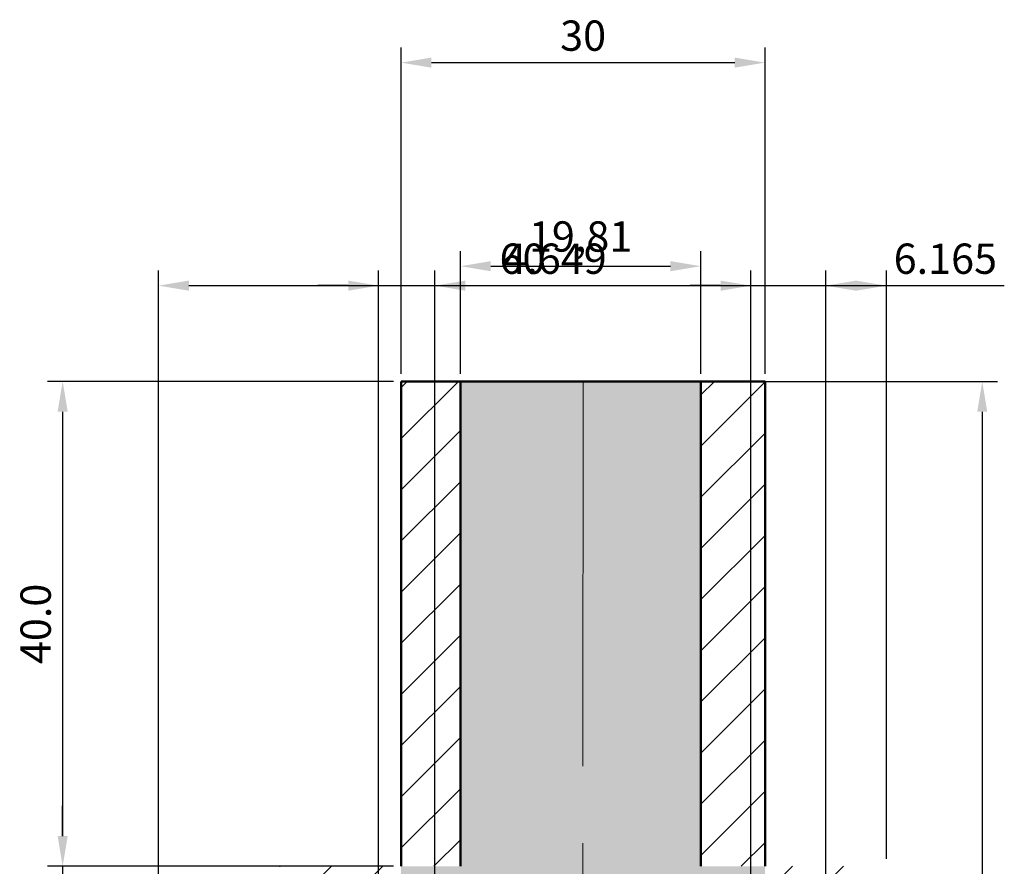
# Model space of a CAD drawing. Units: millimetres. Extents: x 1159 to 1466, y 1237 to 1440.
# Tile 6 of 6: x 1378 to 1459, y 1336 to 1405. Entities that reach past the tile are written whole.
import ezdxf

# ---------------------------------------------------------------- set-up
doc = ezdxf.new("R2010")
doc.units = ezdxf.units.MM
doc.linetypes.add('CENTER', pattern=[50.8, 31.75, -6.35, 6.35, -6.35])
for name, color, linetype, lineweight in [('M-CNTR', 1, 'CENTER', 18), ('M-DIMS', 2, 'Continuous', 25), ('M-HATC', 8, 'Continuous', 18), ('M-OUTL', 7, 'Continuous', 50)]:
    doc.layers.add(name, color=color, linetype=linetype, lineweight=lineweight)
doc.styles.get("Standard").update_dxf_attribs({"font": 'arial.ttf'})
doc.dimstyles.new('ISO-25', dxfattribs={"dimtxt": 2.5, "dimasz": 2.5, "dimexe": 1.25, "dimexo": 0.625, "dimtad": 1, "dimtxsty": 'Standard', "dimcen": 2.5, "dimadec": 0, "dimazin": 0, "dimtfac": 1, "dimtmove": 0, "dimatfit": 3, "dimfxl": 1, "dimarcsym": 0})

# ---------------------------------------------------------------- blocks, each defined once
blk = doc.blocks.new('*D20')
at = {"layer": 'Defpoints', "color": 0, "transparency": 16777216}
for p in [(1439.751, 1401.86), (1409.751, 1375.561), (1439.751, 1375.561)]:
    blk.add_point(p, dxfattribs=at)
at = {"layer": 'M-DIMS', "color": 0, "lineweight": -2, "transparency": 16777216}
for p, q in [((1409.751, 1376.186), (1409.751, 1403.11)), ((1439.751, 1376.186), (1439.751, 1403.11)), ((1412.251, 1401.86), (1437.251, 1401.86))]:
    blk.add_line(p, q, dxfattribs=at)
at = {"layer": 'M-DIMS', "color": 0, "transparency": 16777216}
for points in [[(1412.251, 1402.277), (1412.251, 1401.443), (1409.751, 1401.86)], [(1437.251, 1402.277), (1437.251, 1401.443), (1439.751, 1401.86)]]:
    blk.add_solid(points, dxfattribs=at)
at = {"layer": 'M-DIMS', "color": 0, "transparency": 16777216, "insert": (1424.751, 1403.762), "char_height": 2.5, "attachment_point": 5}
blk.add_mtext('30', dxfattribs=at)
blk = doc.blocks.new('*D21')
at = {"layer": 'Defpoints', "color": 0, "transparency": 16777216}
for p in [(1434.452, 1385.066), (1414.637, 1375.561), (1434.452, 1375.561)]:
    blk.add_point(p, dxfattribs=at)
at = {"layer": 'M-DIMS', "color": 0, "lineweight": -2, "transparency": 16777216}
for p, q in [((1414.637, 1376.186), (1414.637, 1386.316)), ((1434.452, 1376.186), (1434.452, 1386.316)), ((1417.137, 1385.066), (1431.952, 1385.066))]:
    blk.add_line(p, q, dxfattribs=at)
at = {"layer": 'M-DIMS', "color": 0, "transparency": 16777216}
for points in [[(1417.137, 1385.483), (1417.137, 1384.649), (1414.637, 1385.066)], [(1431.952, 1385.483), (1431.952, 1384.649), (1434.452, 1385.066)]]:
    blk.add_solid(points, dxfattribs=at)
at = {"layer": 'M-DIMS', "color": 0, "transparency": 16777216, "insert": (1424.544, 1387.193), "char_height": 2.5, "attachment_point": 5}
blk.add_mtext('19,81', dxfattribs=at)
blk = doc.blocks.new('*D42')
at = {"layer": 'Defpoints', "color": 0, "transparency": 16777216}
for p in [(1409.751, 1375.561), (1424.964, 1255.799), (1457.651, 1255.799)]:
    blk.add_point(p, dxfattribs=at)
at = {"layer": 'M-DIMS', "color": 0, "lineweight": -2, "transparency": 16777216}
for p, q in [((1410.376, 1375.561), (1458.901, 1375.561)), ((1457.651, 1373.061), (1457.651, 1258.299)), ((1425.589, 1255.799), (1458.901, 1255.799))]:
    blk.add_line(p, q, dxfattribs=at)
at = {"layer": 'M-DIMS', "color": 0, "transparency": 16777216}
for points in [[(1457.234, 1373.061), (1458.067, 1373.061), (1457.651, 1375.561)], [(1457.234, 1258.299), (1458.067, 1258.299), (1457.651, 1255.799)]]:
    blk.add_solid(points, dxfattribs=at)
at = {"layer": 'M-DIMS', "color": 0, "transparency": 16777216, "insert": (1455.749, 1315.68), "char_height": 2.5, "attachment_point": 5, "rotation": 90}
blk.add_mtext('119.76', dxfattribs=at)
blk = doc.blocks.new('*D43')
at = {"layer": 'Defpoints', "color": 0, "transparency": 16777216}
for p in [(1449.751, 1383.461), (1449.751, 1335.561), (1389.751, 1330.561)]:
    blk.add_point(p, dxfattribs=at)
at = {"layer": 'M-DIMS', "color": 0, "lineweight": -2, "transparency": 16777216}
for p, q in [((1389.751, 1331.186), (1389.751, 1384.711)), ((1449.751, 1336.186), (1449.751, 1384.711)), ((1392.251, 1383.461), (1447.251, 1383.461))]:
    blk.add_line(p, q, dxfattribs=at)
at = {"layer": 'M-DIMS', "color": 0, "transparency": 16777216}
for points in [[(1392.251, 1383.878), (1392.251, 1383.044), (1389.751, 1383.461)], [(1447.251, 1383.878), (1447.251, 1383.044), (1449.751, 1383.461)]]:
    blk.add_solid(points, dxfattribs=at)
at = {"layer": 'M-DIMS', "color": 0, "transparency": 16777216, "insert": (1419.751, 1385.362), "char_height": 2.5, "attachment_point": 5}
blk.add_mtext('60', dxfattribs=at)
blk = doc.blocks.new('*D57')
at = {"layer": 'Defpoints', "color": 0, "transparency": 16777216}
for p in [(1409.751, 1375.561), (1381.851, 1335.561), (1409.751, 1335.561)]:
    blk.add_point(p, dxfattribs=at)
at = {"layer": 'M-DIMS', "color": 0, "lineweight": -2, "transparency": 16777216}
for p, q in [((1409.126, 1375.561), (1380.601, 1375.561)), ((1381.851, 1373.061), (1381.851, 1338.061)), ((1409.126, 1335.561), (1380.601, 1335.561))]:
    blk.add_line(p, q, dxfattribs=at)
at = {"layer": 'M-DIMS', "color": 0, "transparency": 16777216}
for points in [[(1381.434, 1373.061), (1382.267, 1373.061), (1381.851, 1375.561)], [(1381.434, 1338.061), (1382.267, 1338.061), (1381.851, 1335.561)]]:
    blk.add_solid(points, dxfattribs=at)
at = {"layer": 'M-DIMS', "color": 0, "transparency": 16777216, "insert": (1379.949, 1355.561), "char_height": 2.5, "attachment_point": 5, "rotation": 90}
blk.add_mtext('40.0', dxfattribs=at)
blk = doc.blocks.new('*D58')
at = {"layer": 'Defpoints', "color": 0, "transparency": 16777216}
for p in [(1399.751, 1335.561), (1381.851, 1330.561), (1389.751, 1330.561)]:
    blk.add_point(p, dxfattribs=at)
at = {"layer": 'M-DIMS', "color": 0, "lineweight": -2, "transparency": 16777216}
for p, q in [((1381.851, 1338.061), (1381.851, 1340.561)), ((1399.126, 1335.561), (1380.601, 1335.561)), ((1381.851, 1335.561), (1381.851, 1330.561)), ((1389.126, 1330.561), (1380.601, 1330.561)), ((1381.851, 1328.061), (1381.851, 1319.768))]:
    blk.add_line(p, q, dxfattribs=at)
at = {"layer": 'M-DIMS', "color": 0, "transparency": 16777216}
for points in [[(1381.434, 1338.061), (1382.267, 1338.061), (1381.851, 1335.561)], [(1381.434, 1328.061), (1382.267, 1328.061), (1381.851, 1330.561)]]:
    blk.add_solid(points, dxfattribs=at)
at = {"layer": 'M-DIMS', "color": 0, "transparency": 16777216, "insert": (1379.949, 1322.665), "char_height": 2.5, "attachment_point": 5, "rotation": 90}
blk.add_mtext('5.0', dxfattribs=at)
blk = doc.blocks.new('*D74')
at = {"layer": 'Defpoints', "color": 0, "transparency": 16777216}
for p in [(1412.534, 1383.461), (1407.885, 1271.665), (1412.534, 1264.983)]:
    blk.add_point(p, dxfattribs=at)
at = {"layer": 'M-DIMS', "color": 0, "lineweight": -2, "transparency": 16777216}
for p, q in [((1407.885, 1272.29), (1407.885, 1384.711)), ((1412.534, 1265.608), (1412.534, 1384.711)), ((1405.385, 1383.461), (1402.885, 1383.461)), ((1407.885, 1383.461), (1412.534, 1383.461)), ((1415.034, 1383.461), (1427.326, 1383.461))]:
    blk.add_line(p, q, dxfattribs=at)
at = {"layer": 'M-DIMS', "color": 0, "transparency": 16777216}
for points in [[(1405.385, 1383.878), (1405.385, 1383.044), (1407.885, 1383.461)], [(1415.034, 1383.878), (1415.034, 1383.044), (1412.534, 1383.461)]]:
    blk.add_solid(points, dxfattribs=at)
at = {"layer": 'M-DIMS', "color": 0, "transparency": 16777216, "insert": (1422.43, 1385.362), "char_height": 2.5, "attachment_point": 5}
blk.add_mtext('4.649', dxfattribs=at)
blk = doc.blocks.new('*D75')
at = {"layer": 'Defpoints', "color": 0, "transparency": 16777216}
for p in [(1444.751, 1383.461), (1444.751, 1270.561), (1438.586, 1264.983)]:
    blk.add_point(p, dxfattribs=at)
at = {"layer": 'M-DIMS', "color": 0, "lineweight": -2, "transparency": 16777216}
for p, q in [((1438.586, 1265.608), (1438.586, 1384.711)), ((1444.751, 1271.186), (1444.751, 1384.711)), ((1436.086, 1383.461), (1433.586, 1383.461)), ((1438.586, 1383.461), (1444.751, 1383.461)), ((1447.251, 1383.461), (1459.469, 1383.461))]:
    blk.add_line(p, q, dxfattribs=at)
at = {"layer": 'M-DIMS', "color": 0, "transparency": 16777216}
for points in [[(1436.086, 1383.878), (1436.086, 1383.044), (1438.586, 1383.461)], [(1447.251, 1383.878), (1447.251, 1383.044), (1444.751, 1383.461)]]:
    blk.add_solid(points, dxfattribs=at)
at = {"layer": 'M-DIMS', "color": 0, "transparency": 16777216, "insert": (1454.61, 1385.362), "char_height": 2.5, "attachment_point": 5}
blk.add_mtext('6.165', dxfattribs=at)

msp = doc.modelspace()

# ---------------------------------------------------------------- hatches: boundary and pattern name
at = {"layer": 'M-HATC'}
h = msp.add_hatch(dxfattribs=at)
h.set_pattern_fill('ANSI31', color=256, scale=0.94)
h.set_pattern_definition([(45, (0, -76.8912), (-2.11036, 2.11036), [])])
h.paths.add_polyline_path([(1414.6374, 1375.561), (1409.7508, 1375.561), (1409.7508, 1335.561), (1414.6374, 1335.561)])
h.paths.add_polyline_path([(1439.7508, 1375.561), (1434.4515, 1375.561), (1434.4515, 1335.561), (1439.7508, 1335.561)])
h.paths.add_polyline_path([(1449.7508, 1315.561), (1444.7508, 1315.561), (1444.7508, 1320.561), (1449.7508, 1320.561), (1449.7508, 1335.561), (1439.7508, 1335.561), (1439.7508, 1320.561), (1429.7508, 1320.561), (1429.7508, 1317.561), (1434.7508, 1317.561), (1434.7508, 1282.561), (1429.7508, 1282.561), (1429.7508, 1267.561, -0.1562704), (1427.7989, 1264.9827), (1438.5857, 1264.9827), (1444.7508, 1270.561), (1444.7508, 1275.561), (1444.7508, 1295.561), (1449.7508, 1295.561)])
h.paths.add_polyline_path([(1414.7508, 1317.561), (1419.7508, 1317.561), (1419.7508, 1320.561), (1409.7508, 1320.561), (1409.7508, 1335.561), (1399.7508, 1335.561), (1399.7508, 1330.561), (1389.7508, 1330.561), (1389.7508, 1320.561), (1399.7508, 1320.561), (1399.7508, 1315.561), (1404.7508, 1315.561), (1407.8849, 1311.6652), (1407.8849, 1301.6652), (1402.8849, 1301.6652), (1402.8849, 1281.6652), (1407.8849, 1281.6652), (1407.8849, 1271.6652), (1412.5343, 1264.9827), (1421.7027, 1264.9827, -0.1562704), (1419.7508, 1267.561), (1419.7508, 1282.561), (1414.7508, 1282.561)])
h.paths.add_polyline_path([(1424.6651, 1264.0191, -0.1502665), (1421.7027, 1264.9827), (1412.5343, 1264.9827), (1415.9205, 1260.1158, 0.2337513), (1424.6588, 1255.7945)])
h.paths.add_polyline_path([(1433.7538, 1260.6108), (1438.5857, 1264.9827), (1427.7989, 1264.9827, -0.1585441), (1424.6651, 1264.0191), (1424.6588, 1255.7945, 0.248431)])
h = msp.add_hatch(color=256, dxfattribs=at)
h.set_gradient(color1=(34, 52, 110), color2=(0, 0, 0))
h.paths.add_polyline_path([(1424.7508, 1375.561), (1414.6374, 1375.561), (1414.6374, 1335.561), (1424.7201, 1335.561)])
h.paths.add_polyline_path([(1434.4515, 1375.561), (1424.7508, 1375.561), (1424.7201, 1335.561), (1434.4515, 1335.561)])
h.paths.add_polyline_path([(1424.7201, 1335.561), (1414.6374, 1335.561), (1409.7508, 1335.561), (1409.7508, 1320.561), (1424.7085, 1320.561)])
h.paths.add_polyline_path([(1439.7508, 1335.561), (1424.7201, 1335.561), (1424.7085, 1320.561), (1424.7508, 1320.561), (1439.7508, 1320.561)])
h.paths.add_polyline_path([(1434.7508, 1317.561), (1429.7508, 1317.561), (1424.7062, 1317.561), (1424.6793, 1282.561), (1424.7508, 1282.561), (1434.7508, 1282.561)])
h.paths.add_polyline_path([(1424.7062, 1317.561), (1419.7508, 1317.561), (1414.7508, 1317.561), (1414.7508, 1282.561), (1424.6793, 1282.561)])
h.paths.add_polyline_path([(1424.6793, 1282.561), (1419.7508, 1282.561), (1419.7508, 1267.561), (1424.6678, 1267.561)])
h.paths.add_polyline_path([(1429.7508, 1282.561), (1424.6793, 1282.561), (1424.6678, 1267.561), (1429.7508, 1267.561)])
h.paths.add_polyline_path([(1424.6678, 1267.561), (1419.7508, 1267.561, 0.2389901), (1424.6658, 1264.9833)])
h.paths.add_polyline_path([(1429.7508, 1267.561), (1424.6678, 1267.561), (1424.6658, 1264.9833, 0.2463189)])
h.paths.add_polyline_path([(1419.7508, 1267.561, 0.1562704), (1421.7027, 1264.9827), (1424.7508, 1264.9827, -0.2426514)])
h.paths.add_polyline_path([(1429.7508, 1267.561, -0.2426514), (1424.7508, 1264.9827), (1427.7989, 1264.9827, 0.1562704)], flags=17)
h.paths.add_polyline_path([(1427.7989, 1264.9827), (1424.7508, 1264.9827), (1424.6658, 1264.9827), (1424.6651, 1264.0191, 0.1585441)])
h.paths.add_polyline_path([(1424.6658, 1264.9827), (1421.7027, 1264.9827, 0.1502665), (1424.6651, 1264.0191)])

# ---------------------------------------------------------------- linework, layer by layer
at = {"layer": 'M-CNTR'}
msp.add_line((1424.7508, 1375.561), (1424.6588, 1255.7945), dxfattribs=at)
at = {"layer": 'M-OUTL'}
for p, q in [((1409.7508, 1375.561), (1439.7508, 1375.561)), ((1409.7508, 1335.561), (1409.7508, 1375.561)), ((1414.6374, 1335.561), (1414.6374, 1375.561)), ((1434.4515, 1375.561), (1434.4515, 1335.561)), ((1439.7508, 1375.561), (1439.7508, 1335.561))]:
    msp.add_line(p, q, dxfattribs=at)

# ---------------------------------------------------------------- dimensions: what is measured, and where the dimension line sits
at = {"layer": 'M-DIMS'}
for base, p1, p2, override, picture, middle in [((1439.7508, 1401.86), (1409.7508, 1375.561), (1439.7508, 1375.561), {"dimclrd": 0, "dimclre": 0, "dimclrt": 0}, '*D20', (1424.7508, 1403.7622)), ((1434.4515, 1385.0659), (1414.6374, 1375.561), (1434.4515, 1375.561), {"dimclrd": 0, "dimclre": 0, "dimclrt": 0}, '*D21', (1424.5445, 1387.1933)), ((1449.7508, 1383.461), (1389.7508, 1330.561), (1449.7508, 1335.561), {"dimdec": 0, "dimlfac": 1, "dimrnd": 0, "dimzin": 0, "dimdsep": 46, "dimlunit": 2}, '*D43', (1419.7508, 1385.3624)), ((1412.5343, 1383.461), (1407.8849, 1271.6652), (1412.5343, 1264.9827), {"dimdec": 3, "dimlfac": 1, "dimrnd": 0, "dimzin": 0, "dimdsep": 46, "dimlunit": 2}, '*D74', (1422.4303, 1385.3624)), ((1444.7508, 1383.461), (1438.5857, 1264.9827), (1444.7508, 1270.561), {"dimdec": 3, "dimlfac": 1, "dimrnd": 0, "dimzin": 0, "dimdsep": 46, "dimlunit": 2}, '*D75', (1454.6101, 1385.3624))]:
    dim = msp.add_linear_dim(base=base, p1=p1, p2=p2, dimstyle='ISO-25', override=override, dxfattribs=at)
    dim.commit()
    dim.dimension.update_dxf_attribs({"geometry": picture, "text_midpoint": middle})
for base, p1, p2, override, picture, middle in [((1381.8508, 1335.561), (1409.7508, 1375.561), (1409.7508, 1335.561), {"dimdec": 1, "dimlfac": 1, "dimrnd": 0, "dimzin": 0, "dimdsep": 46, "dimlunit": 2}, '*D57', (1379.9494, 1355.561)), ((1457.6508, 1255.7988), (1409.7508, 1375.561), (1424.9638, 1255.7988), {"dimdec": 2, "dimlfac": 1, "dimrnd": 0, "dimzin": 0, "dimdsep": 46, "dimlunit": 2}, '*D42', (1455.7494, 1315.6799)), ((1381.8508, 1330.561), (1399.7508, 1335.561), (1389.7508, 1330.561), {"dimdec": 1, "dimlfac": 1, "dimrnd": 0, "dimzin": 0, "dimdsep": 46, "dimlunit": 2}, '*D58', (1379.9494, 1322.6645))]:
    dim = msp.add_linear_dim(base=base, p1=p1, p2=p2, angle=90, dimstyle='ISO-25', override=override, dxfattribs=at)
    dim.commit()
    dim.dimension.update_dxf_attribs({"geometry": picture, "text_midpoint": middle})

doc.saveas('drawing.dxf')
